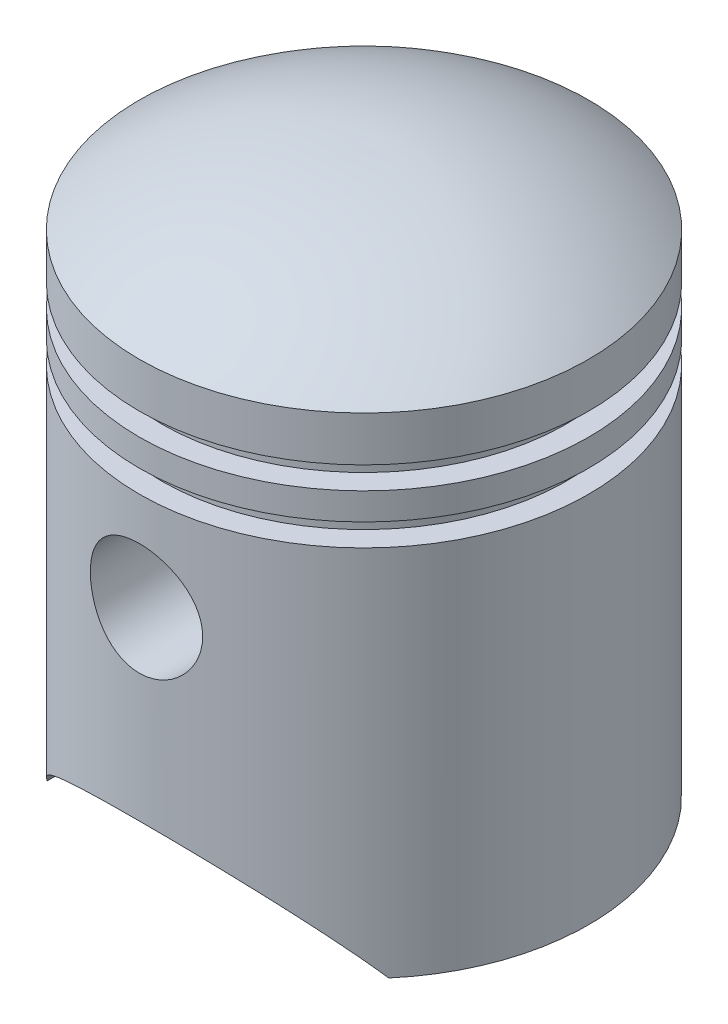
SolidWorks part; units mm, degrees
material "Plain Carbon Steel"
ref_plane "Front Plane" through (0, 0, 0) normal (0, 0, 1) x (1, 0, 0)
ref_plane "Top Plane" through (0, 0, 0) normal (0, 1, 0) x (1, 0, 0)
ref_plane "Right Plane" through (0, 0, 0) normal (1, 0, 0) x (0, 0, -1)
sketch "Piston Profile Sketch" plane through (0, 0, 0) normal (0, 0, 1) x (1, 0, 0)
  line L0 (25, 0) -> (25, 41.5)
  line L1 (25, 49.5) -> (22.5, 49.5)
  line L2 (22.5, 49.5) -> (22.5, 47)
  line L3 (22.5, 47) -> (25, 47)
  line L4 (25, 44) -> (22.5, 44)
  line L5 (22.5, 44) -> (22.5, 41.5)
  line L6 (22.5, 41.5) -> (25, 41.5)
  line L7 (25, 49.5) -> (25, 54.5)
  line L8 (25, 44) -> (25, 47)
  line L9 (23, 0) -> (23, 39.5)
  line L10 (20.5, 39.5) -> (23, 39.5)
  line L11 (20.5, 45.5) -> (20.5, 39.5)
  line L12 (20.5, 45.5) -> (20.5, 45.5)
  line L13 (20.5, 45.5) -> (20.5, 45.5)
  line L14 (20.5, 45.5) -> (20.5, 45.5)
  line L15 (20.5, 51.5) -> (20.5, 45.5)
  line L16 (23, 51.5) -> (20.5, 51.5)
  line L17 (23, 51.5) -> (23, 53.4845)
  line L20 (0, 62.5) -> (0, 60.4994)
  line L21 (25, 0) -> (23, 0)
  arc A0 (25, 54.5) -> (0, 62.5) centre (0.9839, 22.5121) ccw
  arc A1 (23, 53.4845) -> (0, 60.4994) centre (0.9839, 22.5121) ccw
  arc A2 (23, 53.4845) -> (0.0492, 60.5006) centre (0.9839, 22.5121) ccw construction
  dimension "D4" = 40
  dimension "D1" = 62.5
  dimension "D2" = 54.5
  dimension "D3" = 25
  dimension "D5" = 2.5
  dimension "D6" = 5
  dimension "D7" = 2.5
  dimension "D8" = 3
  dimension "D9" = 2.5
  dimension "D10" = 2
revolve "Piston Body with Ring Grooves" add sketch "Piston Profile Sketch" angle 360 about L20
sketch "Skirt Relief Sketch" plane through (0, 0, 0) normal (0, 0, 1) x (1, 0, 0)
  line L0 (-25, 0) -> (25, 0) construction
  line L1 (0, 30.5) -> (0, 62.5) construction
  line L2 (-19, 0) -> (19, 0)
  circle A0 centre (0, 30.5) radius 6.25
  arc A1 (-19, 0) -> (19, 0) centre (0, -13.05) cw
  point P5 (0, 10)
  dimension "D1" = 12.5
  dimension "D2" = 32
  dimension "D3" = 38
  dimension "D4" = 10
extrude "Skirt Relief Cut" cut sketch "Skirt Relief Sketch" against normal through all both and the other way through all
sketch "Pin Boss Sketch" plane through (0, 0, 0) normal (0, 0, 1) x (1, 0, 0)
  circle A0 centre (0, 30.5) radius 7.25
  circle A1 centre (0, 30.5) radius 6.25
  dimension "D1" = 14.5
  dimension "D2" = 12.5
extrude "Pin Boss" add sketch "Pin Boss Sketch" along normal up to surface (11.9257 mm away) from offset 12
mirror "Pin Boss Mirror" about plane through (0, 0, 0) normal (0, 0, 1) of "Pin Boss"
